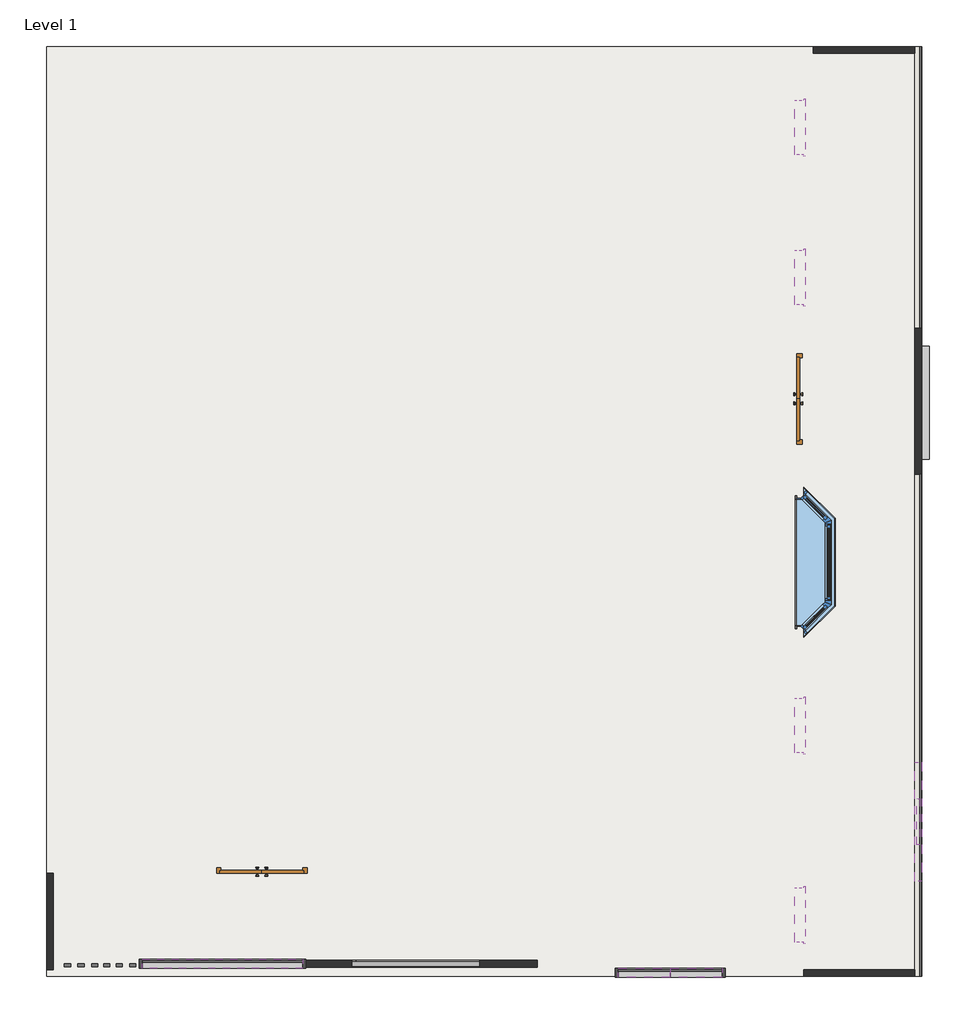
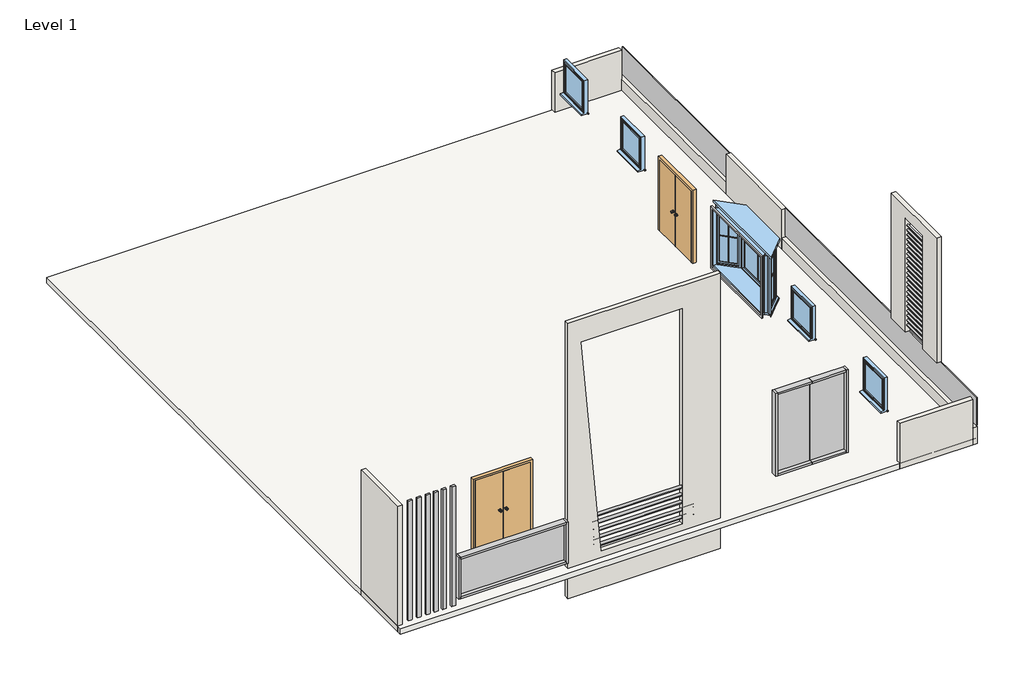
# One storey: 10 members, 8 proxies, 8 walls, 5 plates, 5 windows, 2 doors, 1 covering.
"""IFC4 building model written with IfcOpenShell, lengths in millimetres."""

from ifc_helpers import new_model, si_unit, frame, origin, place, context, project, spatial, polyline, outline, extrude, faceted_brep, transform, mapped, element, save
from components import generic_models_10_generic_models_10_d23db068, generic_models_5_generic_models_5_60d6e435, generic_models_6_generic_models_2_9af304e7, generic_models_9_generic_models_9_b27368f7, muntin_pattern_2x2_muntin_pattern_2x2_511ed329, muntin_pattern_2x2_muntin_pattern_2x2_63bd3b25, trim_window_interior_flat_picture_frame_e25f2530, doors_extdbl_flush_1510x2110mm_6aadbff8, rectangular_mullion_50x150mm_8753fc4c, rectangular_mullion_50x150mm_5ffedf64, rectangular_mullion_50x150mm_024f1578, rectangular_mullion_50x150mm_5671121a, system_panel_glazed_c09e287b, system_panel_glazed_a729a16e, system_panel_glazed_a1088a40, system_panel_glazed_4881c73b, window_f0ba1490, windows_sgl_plain_910x910mm_53772929

model = new_model("IFC4")

# Units and contexts
model_context = context("Model", 3, world=origin())
ifc_project = project(units=[si_unit("LENGTHUNIT", "METRE", prefix="MILLI")], contexts=[model_context])

# Site, building, storey
site = spatial("IfcSite", under=ifc_project)
building = spatial("IfcBuilding", under=site)
storey = spatial("IfcBuildingStorey", under=building, Name="Level 1", Elevation=3352.8)

# Proxies
placement = place(None, origin())
generic_models_10_generic_models_10_shape = generic_models_10_generic_models_10_d23db068(model_context)
element("IfcBuildingElementProxy", 1, Name="Generic Models 10 : Generic Models 10", ObjectType="Generic Models 10 : Generic Models 10", at=placement, inside=storey, context=model_context, shape_type="MappedRepresentation", body=[
    mapped(generic_models_10_generic_models_10_shape, transform((0.0, 0.0, 0.0), x_axis=(1.0, 0.0, 0.0), y_axis=(0.0, 1.0, 0.0), z_axis=(0.0, 0.0, 1.0))),
])
generic_models_5_generic_models_5_shape = generic_models_5_generic_models_5_60d6e435(model_context)
element("IfcBuildingElementProxy", 2, Name="Generic Models 5 : Generic Models 5", ObjectType="Generic Models 5 : Generic Models 5", at=placement, inside=storey, context=model_context, shape_type="MappedRepresentation", body=[
    mapped(generic_models_5_generic_models_5_shape, transform((0.0, 0.0, 0.0), x_axis=(1.0, 0.0, 0.0), y_axis=(0.0, 1.0, 0.0), z_axis=(0.0, 0.0, 1.0))),
])
generic_models_6_generic_models_2_shape = generic_models_6_generic_models_2_9af304e7(model_context)
element("IfcBuildingElementProxy", 3, Name="Generic Models 6 : Generic Models 2", ObjectType="Generic Models 6 : Generic Models 2", at=placement, inside=storey, context=model_context, shape_type="MappedRepresentation", body=[
    mapped(generic_models_6_generic_models_2_shape, transform((304.8, 88.9, -3154.981126), x_axis=(1.0, 0.0, 0.0), y_axis=(0.0, 1.0, 0.0), z_axis=(0.0, 0.0, 1.0))),
])
generic_models_9_generic_models_9_shape = generic_models_9_generic_models_9_b27368f7(model_context)
element("IfcBuildingElementProxy", 4, Name="Generic Models 9 : Generic Models 9", ObjectType="Generic Models 9 : Generic Models 9", at=placement, inside=storey, context=model_context, shape_type="MappedRepresentation", body=[
    mapped(generic_models_9_generic_models_9_shape, transform((0.0, 0.0, 0.0), x_axis=(1.0, 0.0, 0.0), y_axis=(0.0, 1.0, 0.0), z_axis=(0.0, 0.0, 1.0))),
])
muntin_pattern_2x2_muntin_pattern_2x2_shape = muntin_pattern_2x2_muntin_pattern_2x2_511ed329(model_context)
element("IfcBuildingElementProxy", 5, Name="Muntin Pattern_2x2 : Muntin Pattern_2x2", ObjectType="Muntin Pattern_2x2 : Muntin Pattern_2x2", at=placement, inside=storey, context=model_context, shape_type="MappedRepresentation", body=[
    mapped(muntin_pattern_2x2_muntin_pattern_2x2_shape, transform((-6373.004089, 2308.5531952, 4083.05), x_axis=(0.0, -1.0, 0.0), y_axis=(1.0, 0.0, 0.0), z_axis=(0.0, 0.0, 1.0))),
])
muntin_pattern_2x2_muntin_pattern_2x2_2_shape = muntin_pattern_2x2_muntin_pattern_2x2_63bd3b25(model_context)
element("IfcBuildingElementProxy", 6, Name="Muntin Pattern_2x2 : Muntin Pattern_2x2", ObjectType="Muntin Pattern_2x2 : Muntin Pattern_2x2", at=placement, inside=storey, context=model_context, shape_type="MappedRepresentation", body=[
    mapped(muntin_pattern_2x2_muntin_pattern_2x2_2_shape, transform((-6600.8997934, 3223.244924, 4083.05), x_axis=(0.707106781186547, -0.7071067811865482, 0.0), y_axis=(0.7071067811865482, 0.707106781186547, 0.0), z_axis=(0.0, 0.0, 1.0))),
])
element("IfcBuildingElementProxy", 7, Name="Muntin Pattern_2x2 : Muntin Pattern_2x2", ObjectType="Muntin Pattern_2x2 : Muntin Pattern_2x2", at=placement, inside=storey, context=model_context, shape_type="MappedRepresentation", body=[
    mapped(muntin_pattern_2x2_muntin_pattern_2x2_2_shape, transform((-6600.8997934, 1393.8614664, 4083.05), x_axis=(-0.7071067811865469, -0.7071067811865482, 0.0), y_axis=(0.7071067811865482, -0.7071067811865469, 0.0), z_axis=(0.0, 0.0, 1.0))),
])
trim_window_interior_flat_picture_frame_shape = trim_window_interior_flat_picture_frame_e25f2530(model_context)
element("IfcBuildingElementProxy", 8, Name="Trim-Window-Interior-Flat : Picture Frame", ObjectType="Trim-Window-Interior-Flat : Picture Frame", at=placement, inside=storey, context=model_context, shape_type="MappedRepresentation", body=[
    mapped(trim_window_interior_flat_picture_frame_shape, transform((-6903.229089, 2308.5531952, 5537.2), x_axis=(0.0, -1.0, 0.0), y_axis=(0.0, 0.0, 1.0), z_axis=(-1.0, 0.0, 0.0))),
])

# Covering
element("IfcCovering", 9, ObjectType="300mm_Generic", at=placement, inside=storey, context=model_context, shape_type="SweptSolid", body=[
    extrude(outline(polyline([(-4880.4966301, 10900.1031952), (-4880.4966301, -4593.8968048), (-19412.729089, -4593.8968048), (-19412.729089, 10900.1031952), (-4880.4966301, 10900.1031952)])), frame((0.0, 0.0, 3352.8), z_axis=(0.0, 0.0, 1.0), x_axis=(1.0, 0.0, 0.0)), (0.0, 0.0, 1.0), 152.4),
])

# Doors
doors_extdbl_flush_1510x2110mm_shape = doors_extdbl_flush_1510x2110mm_6aadbff8(model_context)
element("IfcDoor", 10, ObjectType="Doors_ExtDbl_Flush : 1510x2110mm", at=placement, inside=storey, context=model_context, shape_type="MappedRepresentation", body=[
    mapped(doors_extdbl_flush_1510x2110mm_shape, transform((-15824.329089, -2815.8968048, 3352.8), x_axis=(1.0, 0.0, 0.0), y_axis=(0.0, 1.0, 0.0), z_axis=(0.0, 0.0, 1.0))),
])
element("IfcDoor", 11, ObjectType="Doors_ExtDbl_Flush : 1510x2110mm", at=placement, inside=storey, context=model_context, shape_type="MappedRepresentation", body=[
    mapped(doors_extdbl_flush_1510x2110mm_shape, transform((-6846.079089, 5032.7031952, 3352.8), x_axis=(0.0, -1.0, 0.0), y_axis=(1.0, 0.0, 0.0), z_axis=(0.0, 0.0, 1.0))),
])

# Members
rectangular_mullion_50x150mm_shape = rectangular_mullion_50x150mm_8753fc4c(model_context)
element("IfcMember", 12, ObjectType="Rectangular Mullion : 50x150mm", at=placement, inside=storey, context=model_context, shape_type="MappedRepresentation", body=[
    mapped(rectangular_mullion_50x150mm_shape, transform((-9930.929089, -4536.7468048, 6486.5021954), x_axis=(-1.0, 0.0, 0.0), y_axis=(0.0, -1.0, 0.0), z_axis=(0.0, 0.0, 1.0))),
])
element("IfcMember", 13, ObjectType="Rectangular Mullion : 50x150mm", at=placement, inside=storey, context=model_context, shape_type="MappedRepresentation", body=[
    mapped(rectangular_mullion_50x150mm_shape, transform((-8102.129089, -4536.7468048, 4267.2), x_axis=(1.0, 0.0, 0.0), y_axis=(0.0, -1.0, 0.0), z_axis=(0.0, 0.0, -1.0))),
])
rectangular_mullion_50x150mm_2_shape = rectangular_mullion_50x150mm_5ffedf64(model_context)
element("IfcMember", 14, ObjectType="Rectangular Mullion : 50x150mm", at=placement, inside=storey, context=model_context, shape_type="MappedRepresentation", body=[
    mapped(rectangular_mullion_50x150mm_2_shape, transform((-8152.129089, -4536.7468048, 6486.5021954), x_axis=(0.0, 0.0, 1.0), y_axis=(0.0, -1.0, 0.0), z_axis=(1.0, 0.0, 0.0))),
])
element("IfcMember", 15, ObjectType="Rectangular Mullion : 50x150mm", at=placement, inside=storey, context=model_context, shape_type="MappedRepresentation", body=[
    mapped(rectangular_mullion_50x150mm_2_shape, transform((-9880.929089, -4536.7468048, 4267.2), x_axis=(0.0, 0.0, -1.0), y_axis=(0.0, -1.0, 0.0), z_axis=(-1.0, 0.0, 0.0))),
])
element("IfcMember", 16, ObjectType="Rectangular Mullion : 50x150mm", at=placement, inside=storey, context=model_context, shape_type="MappedRepresentation", body=[
    mapped(rectangular_mullion_50x150mm_2_shape, transform((-9016.529089, -4536.7468048, 6486.5021954), x_axis=(0.0, 0.0, 1.0), y_axis=(0.0, -1.0, 0.0), z_axis=(1.0, 0.0, 0.0))),
])
element("IfcMember", 17, ObjectType="Rectangular Mullion : 50x150mm", at=placement, inside=storey, context=model_context, shape_type="MappedRepresentation", body=[
    mapped(rectangular_mullion_50x150mm_2_shape, transform((-9016.529089, -4536.7468048, 4267.2), x_axis=(0.0, 0.0, -1.0), y_axis=(0.0, -1.0, 0.0), z_axis=(-1.0, 0.0, 0.0))),
])
rectangular_mullion_50x150mm_3_shape = rectangular_mullion_50x150mm_024f1578(model_context)
element("IfcMember", 18, ObjectType="Rectangular Mullion : 50x150mm", at=placement, inside=storey, context=model_context, shape_type="MappedRepresentation", body=[
    mapped(rectangular_mullion_50x150mm_3_shape, transform((-17863.329089, -4383.6602029, 4769.818874), x_axis=(-1.0, 0.0, 0.0), y_axis=(0.0, -1.0, 0.0), z_axis=(0.0, 0.0, 1.0))),
])
element("IfcMember", 19, ObjectType="Rectangular Mullion : 50x150mm", at=placement, inside=storey, context=model_context, shape_type="MappedRepresentation", body=[
    mapped(rectangular_mullion_50x150mm_3_shape, transform((-15088.379089, -4383.6602029, 3657.6), x_axis=(1.0, 0.0, 0.0), y_axis=(0.0, -1.0, 0.0), z_axis=(0.0, 0.0, -1.0))),
])
rectangular_mullion_50x150mm_4_shape = rectangular_mullion_50x150mm_5671121a(model_context)
element("IfcMember", 20, ObjectType="Rectangular Mullion : 50x150mm", at=placement, inside=storey, context=model_context, shape_type="MappedRepresentation", body=[
    mapped(rectangular_mullion_50x150mm_4_shape, transform((-15138.379089, -4383.6602029, 4769.818874), x_axis=(0.0, 0.0, 1.0), y_axis=(0.0, -1.0, 0.0), z_axis=(1.0, 0.0, 0.0))),
])
element("IfcMember", 21, ObjectType="Rectangular Mullion : 50x150mm", at=placement, inside=storey, context=model_context, shape_type="MappedRepresentation", body=[
    mapped(rectangular_mullion_50x150mm_4_shape, transform((-17813.329089, -4383.6602029, 3657.6), x_axis=(0.0, 0.0, -1.0), y_axis=(0.0, -1.0, 0.0), z_axis=(-1.0, 0.0, 0.0))),
])

# Plates
system_panel_glazed_shape = system_panel_glazed_c09e287b(model_context)
element("IfcPlate", 22, ObjectType="System Panel : Glazed", at=placement, inside=storey, context=model_context, shape_type="MappedRepresentation", body=[
    mapped(system_panel_glazed_shape, transform((-9448.729089, -4536.7468048, 4317.2), x_axis=(1.0, 0.0, 0.0), y_axis=(0.0, 1.0, 0.0), z_axis=(0.0, 0.0, 1.0))),
])
element("IfcPlate", 23, ObjectType="System Panel : Glazed", at=placement, inside=storey, context=model_context, shape_type="MappedRepresentation", body=[
    mapped(system_panel_glazed_shape, transform((-8584.329089, -4536.7468048, 4317.2), x_axis=(1.0, 0.0, 0.0), y_axis=(0.0, 1.0, 0.0), z_axis=(0.0, 0.0, 1.0))),
])
system_panel_glazed_2_shape = system_panel_glazed_a729a16e(model_context)
element("IfcPlate", 24, ObjectType="System Panel : Glazed", at=placement, inside=storey, context=model_context, shape_type="MappedRepresentation", body=[
    mapped(system_panel_glazed_2_shape, transform((-16475.854089, -4383.6602029, 3707.6), x_axis=(1.0, 0.0, 0.0), y_axis=(0.0, 1.0, 0.0), z_axis=(0.0, 0.0, 1.0))),
])
system_panel_glazed_3_shape = system_panel_glazed_a1088a40(model_context)
element("IfcPlate", 25, ObjectType="System Panel : Glazed", at=placement, inside=storey, context=model_context, shape_type="MappedRepresentation", body=[
    mapped(system_panel_glazed_3_shape, transform((-4880.4966301, 8560.1281952, 3840.4601563), x_axis=(0.0, -1.0, 0.0), y_axis=(1.0, 0.0, 0.0), z_axis=(0.0, 0.0, 1.0))),
])
system_panel_glazed_4_shape = system_panel_glazed_4881c73b(model_context)
element("IfcPlate", 26, ObjectType="System Panel : Glazed", at=placement, inside=storey, context=model_context, shape_type="MappedRepresentation", body=[
    mapped(system_panel_glazed_4_shape, transform((-4880.4966301, -409.2468048, 3840.4601563), x_axis=(0.0, -1.0, 0.0), y_axis=(1.0, 0.0, 0.0), z_axis=(0.0, 0.0, 1.0))),
])

# Walls
element("IfcWall", 27, ObjectType="basic wall", at=placement, inside=storey, context=model_context, shape_type="SweptSolid", body=[
    extrude(outline(polyline([(-19412.729089, -4479.5968048), (-19412.729089, -2873.0468048), (-19298.429089, -2873.0468048), (-19298.429089, -4479.5968048), (-19412.729089, -4479.5968048)])), frame((0.0, 0.0, 3352.8), z_axis=(0.0, 0.0, 1.0), x_axis=(1.0, 0.0, 0.0)), (0.0, 0.0, 1.0), 3352.8),
])
element("IfcWall", 28, ObjectType="basic wall", at=placement, inside=storey, context=model_context, shape_type="Brep", body=[
    faceted_brep([(-4937.6466301, 6213.8031952, 3352.8), (-4937.6466301, 3775.4031952, 3352.8), (-4937.6466301, 3775.4031952, 3810.0), (-4937.6466301, 3775.4031952, 4572.0), (-4937.6466301, 6213.8031952, 4572.0), (-4937.6466301, 6213.8031952, 3810.0), (-4823.3466301, 6213.8031952, 3352.8), (-4823.3466301, 6213.8031952, 3810.0), (-4823.3466301, 6213.8031952, 4572.0), (-4823.3466301, 3775.4031952, 4572.0), (-4823.3466301, 3775.4031952, 3810.0), (-4823.3466301, 3775.4031952, 3352.8)], [[[0, 1, 2, 3, 4, 5]], [[6, 7, 8, 9, 10, 11]], [[1, 0, 6, 11]], [[3, 2, 1, 11, 10, 9]], [[4, 3, 9, 8]], [[0, 5, 4, 8, 7, 6]]]),
])
element("IfcWall", 29, ObjectType="basic wall", at=placement, inside=storey, context=model_context, shape_type="Brep", body=[
    faceted_brep([(-4823.3466301, 6213.8031952, 3352.8), (-4823.3466301, 10906.4531952, 3352.8), (-4823.3466301, 10906.4531952, 3810.0), (-4823.3466301, 6213.8031952, 3810.0), (-4937.6466301, 6213.8031952, 3352.8), (-4937.6466301, 6213.8031952, 3810.0), (-4937.6466301, 10906.4531952, 3810.0), (-4937.6466301, 10906.4531952, 3352.8), (-4937.6466301, 10792.1531952, 3352.8)], [[[0, 1, 2, 3]], [[4, 5, 6, 7, 8]], [[1, 0, 4, 8, 7]], [[3, 2, 6, 5]], [[0, 3, 5, 4]], [[2, 1, 7, 6]]]),
])
element("IfcWall", 30, ObjectType="basic wall", at=placement, inside=storey, context=model_context, shape_type="Brep", body=[
    faceted_brep([(-4937.6466301, 3775.4031952, 3352.8), (-4937.6466301, -4479.5968048, 3352.8), (-4937.6466301, -4593.8968048, 3352.8), (-4937.6466301, -4593.8968048, 3810.0), (-4937.6466301, 3775.4031952, 3810.0), (-4823.3466301, 3775.4031952, 3352.8), (-4823.3466301, 3775.4031952, 3810.0), (-4823.3466301, -4593.8968048, 3810.0), (-4823.3466301, -4593.8968048, 3352.8)], [[[0, 1, 2, 3, 4]], [[5, 6, 7, 8]], [[2, 1, 0, 5, 8]], [[4, 3, 7, 6]], [[0, 4, 6, 5]], [[3, 2, 8, 7]]]),
])
element("IfcWall", 31, ObjectType="basic wall", at=placement, inside=storey, context=model_context, shape_type="Brep", body=[
    faceted_brep([(-4937.6466301, -4479.5968048, 3352.8), (-6788.929089, -4479.5968048, 3352.8), (-6788.929089, -4479.5968048, 4572.0), (-4937.6466301, -4479.5968048, 4572.0), (-4937.6466301, -4593.8968048, 3352.8), (-4937.6466301, -4593.8968048, 3810.0), (-4937.6466301, -4593.8968048, 4572.0), (-6788.929089, -4593.8968048, 4572.0), (-6788.929089, -4593.8968048, 3355.2103724), (-6788.929089, -4593.8968048, 3352.8)], [[[0, 1, 2, 3]], [[4, 5, 6, 7, 8, 9]], [[1, 0, 4, 9]], [[3, 2, 7, 6]], [[2, 1, 9, 8, 7]], [[0, 3, 6, 5, 4]]]),
])
element("IfcWall", 32, ObjectType="basic wall", at=placement, inside=storey, context=model_context, shape_type="Brep", body=[
    faceted_brep([(-4937.6466301, 10906.4531952, 3352.8), (-6630.5177331, 10906.4531952, 3352.8), (-6630.5177331, 10906.4531952, 4572.0), (-4937.6466301, 10906.4531952, 4572.0), (-4937.6466301, 10906.4531952, 3810.0), (-4937.6466301, 10792.1531952, 3352.8), (-4937.6466301, 10792.1531952, 4572.0), (-6630.5177331, 10792.1531952, 4572.0), (-6630.5177331, 10792.1531952, 3352.8)], [[[0, 1, 2, 3, 4]], [[5, 6, 7, 8]], [[1, 0, 5, 8]], [[2, 1, 8, 7]], [[3, 2, 7, 6]], [[0, 4, 3, 6, 5]]]),
])
element("IfcWall", 33, ObjectType="basic wall", at=placement, inside=storey, context=model_context, shape_type="SweptSolid", body=[
    extrude(outline(polyline([(-3006.3968048, 7924.8), (-1025.1968048, 7924.8), (-1025.1968048, 4577.8), (-1634.7968048, 4577.8), (-1634.7968048, 7620.0), (-2396.7968048, 7620.0), (-2396.7968048, 4577.8), (-3006.3968048, 4577.8), (-3006.3968048, 7924.8)])), frame((-4937.6466301, 0.0, 0.0), z_axis=(1.0, 0.0, 0.0), x_axis=(0.0, 1.0, 0.0)), (0.0, 0.0, 1.0), 114.3),
])
element("IfcWall", 34, ObjectType="basic wall 5", at=placement, inside=storey, context=model_context, shape_type="Brep", body=[
    faceted_brep([(-15088.379089, -4438.9224035, 2700.0), (-11233.929089, -4438.9224035, 2700.0), (-11233.929089, -4438.9224035, 6705.6), (-11233.929089, -4438.9224035, 7924.8), (-11233.929089, -4438.9224035, 10058.4), (-15088.379089, -4438.9224035, 10058.4), (-14755.829089, -4438.9224035, 9450.0), (-12191.079089, -4438.9224035, 9450.0), (-12191.079089, -4438.9224035, 3680.8372644), (-14251.0927516, -4438.9224035, 3680.8372644), (-15088.379089, -4324.6224035, 2700.0), (-15088.379089, -4324.6224035, 10058.4), (-11233.929089, -4324.6224035, 10058.4), (-11233.929089, -4324.6224035, 2700.0), (-14755.829089, -4324.6224035, 9450.0), (-14251.0927516, -4324.6224035, 3680.8372644), (-12191.079089, -4324.6224035, 3680.8372644), (-12191.079089, -4324.6224035, 9450.0)], [[[0, 1, 2, 3, 4, 5], [6, 7, 8, 9]], [[10, 11, 12, 13], [14, 15, 16, 17]], [[1, 0, 10, 13]], [[5, 4, 12, 11]], [[0, 5, 11, 10]], [[7, 6, 14, 17]], [[8, 7, 17, 16]], [[9, 8, 16, 15]], [[6, 9, 15, 14]], [[4, 3, 2, 1, 13, 12]]]),
])

# Windows
window_shape = window_f0ba1490(model_context)
element("IfcWindow", 35, ObjectType="Window-Bay-Casement-45_Degree_Angle : 84\" x 60\" x 18\"", at=placement, inside=storey, context=model_context, shape_type="MappedRepresentation", body=[
    mapped(window_shape, transform((-6846.079089, 2308.5531952, 3352.8), x_axis=(0.0, -1.0, 0.0), y_axis=(1.0, 0.0, 0.0), z_axis=(0.0, 0.0, 1.0))),
])
windows_sgl_plain_910x910mm_shape = windows_sgl_plain_910x910mm_53772929(model_context)
element("IfcWindow", 36, ObjectType="Windows_Sgl_Plain : 910x910mm", at=placement, inside=storey, context=model_context, shape_type="MappedRepresentation", body=[
    mapped(windows_sgl_plain_910x910mm_shape, transform((-6837.6225212, -413.3968048, 3352.8), x_axis=(0.0, 1.0, 0.0), y_axis=(-1.0, 0.0, 0.0), z_axis=(0.0, 0.0, 1.0))),
])
element("IfcWindow", 37, ObjectType="Windows_Sgl_Plain : 910x910mm", at=placement, inside=storey, context=model_context, shape_type="MappedRepresentation", body=[
    mapped(windows_sgl_plain_910x910mm_shape, transform((-6837.6225212, -3567.3968048, 3352.8), x_axis=(0.0, 1.0, 0.0), y_axis=(-1.0, 0.0, 0.0), z_axis=(0.0, 0.0, 1.0))),
])
element("IfcWindow", 38, ObjectType="Windows_Sgl_Plain : 910x910mm", at=placement, inside=storey, context=model_context, shape_type="MappedRepresentation", body=[
    mapped(windows_sgl_plain_910x910mm_shape, transform((-6837.6225212, 7058.3531952, 3352.8), x_axis=(0.0, 1.0, 0.0), y_axis=(-1.0, 0.0, 0.0), z_axis=(0.0, 0.0, 1.0))),
])
element("IfcWindow", 39, ObjectType="Windows_Sgl_Plain : 910x910mm", at=placement, inside=storey, context=model_context, shape_type="MappedRepresentation", body=[
    mapped(windows_sgl_plain_910x910mm_shape, transform((-6837.6225212, 9553.9031952, 3352.8), x_axis=(0.0, 1.0, 0.0), y_axis=(-1.0, 0.0, 0.0), z_axis=(0.0, 0.0, 1.0))),
])

save(model, "model.ifc")

# Revit data of these elements
# Type "Muntin Pattern_2x2 : Muntin Pattern_2x2"
#   Width [instance default] = 4' - 0"
#   Thickness = 0' - 0 1/2"
#   Height [instance default] = 4' - 0"
#   Distance = 0' - 0 3/4"
#   Interior Material [instance default] = none
#   Exterior Material [instance default] = none
#   Default Elevation = 0
# Type "Trim-Window-Interior-Flat : Picture Frame"
#   Trim Thickness_Picture Frame = 0' - 1 1/4"
#   Trim Width = 0' - 2 1/4"
#   Trim Thickness_with Sill = 0' - 0 3/4"
#   Sill Thickness = 0' - 1 1/4"
#   Opening Width [instance default] = 2' - 0"
#   Opening Height [instance default] = 3' - 0"
#   Default Elevation = 4' - 0"
#   Sill = no
#   Picture Frame = yes
#   Trim Material [instance default] = none
# Type "300mm_Generic"
#   built-in parameter 1002203 = 1 (stored number, unit not read)
#   built-in parameter 1002202 = 1 (stored number, unit not read)
#   Layers, outside or top first: 0' - 6" no material (function 1)
# Type "Doors_ExtDbl_Flush : 1510x2110mm"
#   Construction Type Id = "MDOOR"
#   Type Mark = "45"
#   Type Comments = "External Double"
#   Operation = "DoubleDoorSingleSwing"
#   Keynote = "L20"
#   Analytic Construction = "Metal"
#   Wrap Layers (Ext) from Ext = 0' - 4.03543"
#   Wrap Layers (Int) from Ext = 0' - 6.98819"
#   Thickness = 0' - 1.73228"
#   Rough Width = 4' - 11.44882"
#   Rough Height = 6' - 11.07087"
#   O/A Frame Width = 0' - 2.51969"
#   Heat Transfer Coefficient (U) = 3.7021 W/(m²·K)
#   Handle Z Distance = 3' - 5.33858"
#   FrameWidth = 0' - 1.65354"
#   FrameOffset - External = 0' - 0.98425"
#   FrameDepth = 0' - 3.50394"
#   Door Panel Width = 2' - 3.6378"
#   Door Panel Thickness = 0' - 1.73228"
#   Door Panel Height = 6' - 6.74016"
#   Cill Thickness = 0' - 2.14567"
#   Cill Projection = 0' - 1.1811"
#   Handle X Distance = 0' - 2.95276"
#   Height = 6' - 11.07087"
#   Structural Tolerance = 0' - 0.25591"
#   Tolerance = 0' - 0.11811"
#   Undercut = 0' - 0.15748"
#   Width = 4' - 11.44882"
#   Cill Extension = 0' - 0.98425"
#   Cavity Closer Width = 0' - 1.9685"
#   Cavity Closer Offset from Ext = 0' - 4.03543"
#   Cavity Closer Depth = 0' - 3.34646"
#   Define Thermal Properties by = 1
#   Vis - Ironmongery = yes
#   Vis - Cavity Closers = yes
#   Function = 1
#   Material Door = Door - Panel
#   Material Frame = Door - Frame/Mullion
#   Material Ironmongery = Door - Handle
#   Visual Light Transmittance = 0
#   Thermal Resistance (R) = 0
#   Solar Heat Gain Coefficient = 0
#   Wall Closure = (empty or 0)
# Type "Rectangular Mullion : 50x150mm"
#   Keynote = "H11"
#   built-in parameter 1007304 = 0.492126 (stored number, unit not read)
#   built-in parameter 1007301 = 0.082021 (stored number, unit not read)
#   built-in parameter 1007300 = 0.082021 (stored number, unit not read)
# Type "System Panel : Glazed"
#   Keynote = "H11"
#   Construction Type Id = "GSP4R"
#   Analytic Construction = "1/8 in Pilkington single glazing"
#   Visual Light Transmittance = 0.9
#   Solar Heat Gain Coefficient = 0.86
#   Heat Transfer Coefficient (U) = 6.7069 W/(m²·K)
#   Define Thermal Properties by = 1
# Type "basic wall"
#   Keynote = "F10"
#   Layers, outside or top first: 0' - 4 1/2" "Air" (function 1)
# Type "basic wall 5"
#   Keynote = "F10"
#   Layers, outside or top first: 0' - 4 1/2" "Roofing, Tile" (function 1)
# Type "Window-Bay-Casement-45_Degree_Angle : 84\" x 60\" x 18\""
#   Type Mark = "50"
#   Fire Rating = "0.5h"
#   Assembly Code = "B2020100"
#   Analytic Construction = "Double glazing - domestic"
#   Width of Middle Sash = 4' - 2.38909"
#   Width = 7' - 0"
#   Visual Light Transmittance = 0.81
#   Thermal Resistance (R) = 0.319569 (m²·K)/W
#   Solar Heat Gain Coefficient = 0.76
#   Rough Width = 7' - 0 1/2"
#   Rough Height = 5' - 0 1/2"
#   Length 4 = 0' - 1.13909"
#   Length 3 = 0' - 0.51777"
#   Length 2 = 4' - 7.42462"
#   Length 1 = 1' - 2.80546"
#   Wall Thickness [instance default] = 0' - 6"
#   Trim Width = 7' - 5.03553"
#   Trim Height = 5' - 0"
#   Height 1 = 5' - 2"
#   Height = 5' - 0"
#   Heat Transfer Coefficient (U) = 3.12929 W/(m²·K)
#   Depth = 1' - 6"
#   Default Sill Height = 2' - 0"
#   Angle 1 = 22.50°
#   Angle = 45.00°
#   Center Muntin Visibility = yes
#   Side Muntin Visibility = yes
#   Interior Trim Visibility [instance default] = yes
#   Exterior Trim Visibility [instance default] = yes
#   Center Muntin Pattern = Muntin Pattern_2x2 : Muntin Pattern_2x2
#   Side Muntin Pattern = Muntin Pattern_2x2 : Muntin Pattern_2x2
#   Interior Trim Material = Wood - Stained
#   Exterior Trim Material = Clad - White
#   Exterior Trim = element 339135
#   Interior Trim = Trim-Window-Interior-Flat : Picture Frame
#   Interior Frame Material = Wood - Stained
#   Glass Panel Material = Glass
#   Exterior Frame Material = Clad - White
#   Wall Closure = (empty or 0)
# Type "Windows_Sgl_Plain : 910x910mm"
#   Type Mark = "44"
#   Operation = "SinglePanel"
#   Construction Type Id = "SGL"
#   Manufacturer = "Revit"
#   Keynote = "L10"
#   Analytic Construction = "Large single-glazed windows"
#   Wrap Layers (Ext) from Ext = 0' - 4.03543"
#   Wrap Layers (Int) from Ext = 0' - 6.98819"
#   Window Board Projection = 0' - 0.98425"
#   Window Board Extension = 0' - 0.98425"
#   Visual Light Transmittance = 0.9
#   Solar Heat Gain Coefficient = 0.86
#   Rough Width = 2' - 11.82677"
#   Rough Height = 2' - 11.82677"
#   Height = 2' - 11.82677"
#   Width = 2' - 11.82677"
#   Heat Transfer Coefficient (U) = 5.5617 W/(m²·K)
#   Glazing Thickness = 0' - 0.94488"
#   FrameOffset - External = 0' - 1.9685"
#   Frame Depth = 0' - 2.55906"
#   Default Head Height = 6' - 11.07087"
#   Cill Depth = 0' - 3.44488"
#   Cavity Closer Width = 0' - 1.9685"
#   Cavity Closer Offset from Ext = 0' - 4.03543"
#   Cavity Closer Depth = 0' - 3.34646"
#   Define Thermal Properties by = 1
#   Vis - Cavity Closers = yes
#   Define Thermal Properties by = 1
#   Material Trim = Window Frame
#   Material Glass = Glass
#   Material Frame = Window Frame
#   Wall Closure = (empty or 0)
# Element 1 (IfcBuildingElementProxy, "Generic Models 10 : Generic Models 10")
#   Phase Created = New Construction
# Element 2 (IfcBuildingElementProxy, "Generic Models 5 : Generic Models 5")
#   Phase Created = New Construction
# Element 3 (IfcBuildingElementProxy, "Generic Models 6 : Generic Models 2")
#   Phase Created = New Construction
# Element 4 (IfcBuildingElementProxy, "Generic Models 9 : Generic Models 9")
#   Phase Created = New Construction
# Element 5 (IfcBuildingElementProxy, "Muntin Pattern_2x2 : Muntin Pattern_2x2")
#   Width = 3' - 8.88909"
#   Height = 4' - 6 1/2"
#   Interior Material = Wood - Stained
#   Exterior Material = Clad - White
#   Phase Created = New Construction
#   Materials on its faces: "Clad - White", "Wood - Stained"
# Elements 6, 7 (IfcBuildingElementProxy, "Muntin Pattern_2x2 : Muntin Pattern_2x2")
#   Width = 1' - 4.18808"
#   Height = 4' - 6 1/2"
#   Interior Material = Wood - Stained
#   Exterior Material = Clad - White
#   Phase Created = New Construction
#   Materials on its faces: "Clad - White", "Wood - Stained"
# Element 8 (IfcBuildingElementProxy, "Trim-Window-Interior-Flat : Picture Frame")
#   Opening Width = 7' - 0"
#   Opening Height = 5' - 2"
#   Trim Material = Wood - Stained
#   Phase Created = New Construction
#   Materials on its faces: "Wood - Stained"
# Element 9 (IfcCovering, "300mm_Generic")
#   Height Offset From Level = 0' - 0"
#   Phase Created = New Construction
#   Materials on its faces: "Default"
# Elements 10, 11 (IfcDoor, "Doors_ExtDbl_Flush : 1510x2110mm")
#   Phase Created = New Construction
#   Materials on its faces: "Door - Handle", "Door - Frame/Mullion", "Door - Panel"
# Elements 12, 13, 14, 15, 16, 17, 18, 19, 20, 21 (IfcMember, "Rectangular Mullion : 50x150mm")
#   Phase Created = New Construction
#   Materials on its faces: "Aluminium"
# Elements 22, 23, 24, 25, 26 (IfcPlate, "System Panel : Glazed")
#   Phase Created = New Construction
#   Materials on its faces: "Glass"
# Element 27 (IfcWall, "basic wall")
#   Top Offset = 0' - 0"
#   Base Offset = 0' - 0"
#   wall height = 11' - 0"
#   Phase Created = New Construction
#   Base Constraint = Level 1
#   Top Constraint = Level 2
#   Materials on its faces: "Air"
# Element 28 (IfcWall, "basic wall")
#   Top Offset = 0' - 0"
#   Base Offset = 0' - 0"
#   Unconnected Height = 4' - 0"
#   wall height = 4' - 0"
#   Phase Created = New Construction
#   Base Constraint = Level 1
#   Materials on its faces: "Air"
# Elements 29, 30 (IfcWall, "basic wall")
#   Top Offset = 0' - 0"
#   Base Offset = 0' - 0"
#   Unconnected Height = 1' - 6"
#   wall height = 1' - 6"
#   Phase Created = New Construction
#   Base Constraint = Level 1
#   Materials on its faces: "Air"
# Elements 31, 32 (IfcWall, "basic wall")
#   Top Offset = 10' - 0"
#   Base Offset = 0' - 0"
#   Unconnected Height = 4' - 0"
#   wall height = 4' - 0"
#   Phase Created = New Construction
#   Base Constraint = Level 1
#   Materials on its faces: "Air"
# Element 33 (IfcWall, "basic wall")
#   built-in parameter 1001111 = 1' - 7 51/256"
#   Top Offset = 10' - 0"
#   Base Offset = 1' - 7 51/256"
#   Unconnected Height = 13' - 4 205/256"
#   wall height = 13' - 4 205/256"
#   Phase Created = New Construction
#   Base Constraint = Level 1
#   Materials on its faces: "Air"
# Element 34 (IfcWall, "basic wall 5")
#   built-in parameter 1001111 = -2' - 1.70079"
#   Top Offset = 0' - 0"
#   Base Offset = -2' - 1.70079"
#   wall height = 24' - 1.70079"
#   Phase Created = New Construction
#   Base Constraint = Level 1
#   Top Constraint = Level 3
#   Materials on its faces: "Roofing, Tile", "Brick, Common"
# Element 35 (IfcWindow, "Window-Bay-Casement-45_Degree_Angle : 84\" x 60\" x 18\"")
#   Mark = "13"
#   Interior Trim Visibility = yes
#   Exterior Trim Visibility = yes
#   Phase Created = New Construction
#   Materials on its faces: "Wood - Stained", "Clad - White", "Glass"
# Element 36 (IfcWindow, "Windows_Sgl_Plain : 910x910mm")
#   Mark = "9"
#   Phase Created = New Construction
#   Materials on its faces: "Window Frame", "Glass"
# Element 37 (IfcWindow, "Windows_Sgl_Plain : 910x910mm")
#   Mark = "10"
#   Phase Created = New Construction
#   Materials on its faces: "Window Frame", "Glass"
# Element 38 (IfcWindow, "Windows_Sgl_Plain : 910x910mm")
#   Mark = "11"
#   Phase Created = New Construction
#   Materials on its faces: "Window Frame", "Glass"
# Element 39 (IfcWindow, "Windows_Sgl_Plain : 910x910mm")
#   Mark = "12"
#   Phase Created = New Construction
#   Materials on its faces: "Window Frame", "Glass"
# Materials
#   "Door - Panel": class "Wood", colour RGB 210 159 95, transparency 0, Keynote = "L20", Cost = 0
#   "Door - Frame/Mullion": class "Wood", colour RGB 212 179 113, transparency 0, Keynote = "L20", Cost = 0
#   "Door - Handle": colour RGB 17 17 17, transparency 0, Keynote = "P21", Cost = 0
#   "Air": class "Gas", colour RGB 255 255 255, transparency 0, Description = "Air", Cost = 0
#   "Roofing, Tile": class "Metal", colour RGB 190 129 78, transparency 0, Description = "Clay roofing tile", Cost = 0
#   "Wood - Stained": class "Wood", colour RGB 227 170 128, transparency 0, Cost = 0
#   "Clad - White": class "Wood", colour RGB 242 242 238, transparency 0, Cost = 0
#   "Glass": class "Glass", colour RGB 0 128 192, transparency 0.9, Description = "Soda Lime Glass", Cost = 0
#   "Window Frame": colour RGB 249 249 249, transparency 0, Keynote = "L10", Cost = 0
#   "Default": colour RGB 127 127 127, transparency 0, Cost = 0
#   "Aluminium": class "Metal", colour RGB 247 247 247, transparency 0, Description = "Aluminium 6061", Cost = 0
#   "Brick, Common": class "Masonry", colour RGB 170 100 105, transparency 0, Description = "Common brick", Cost = 0
